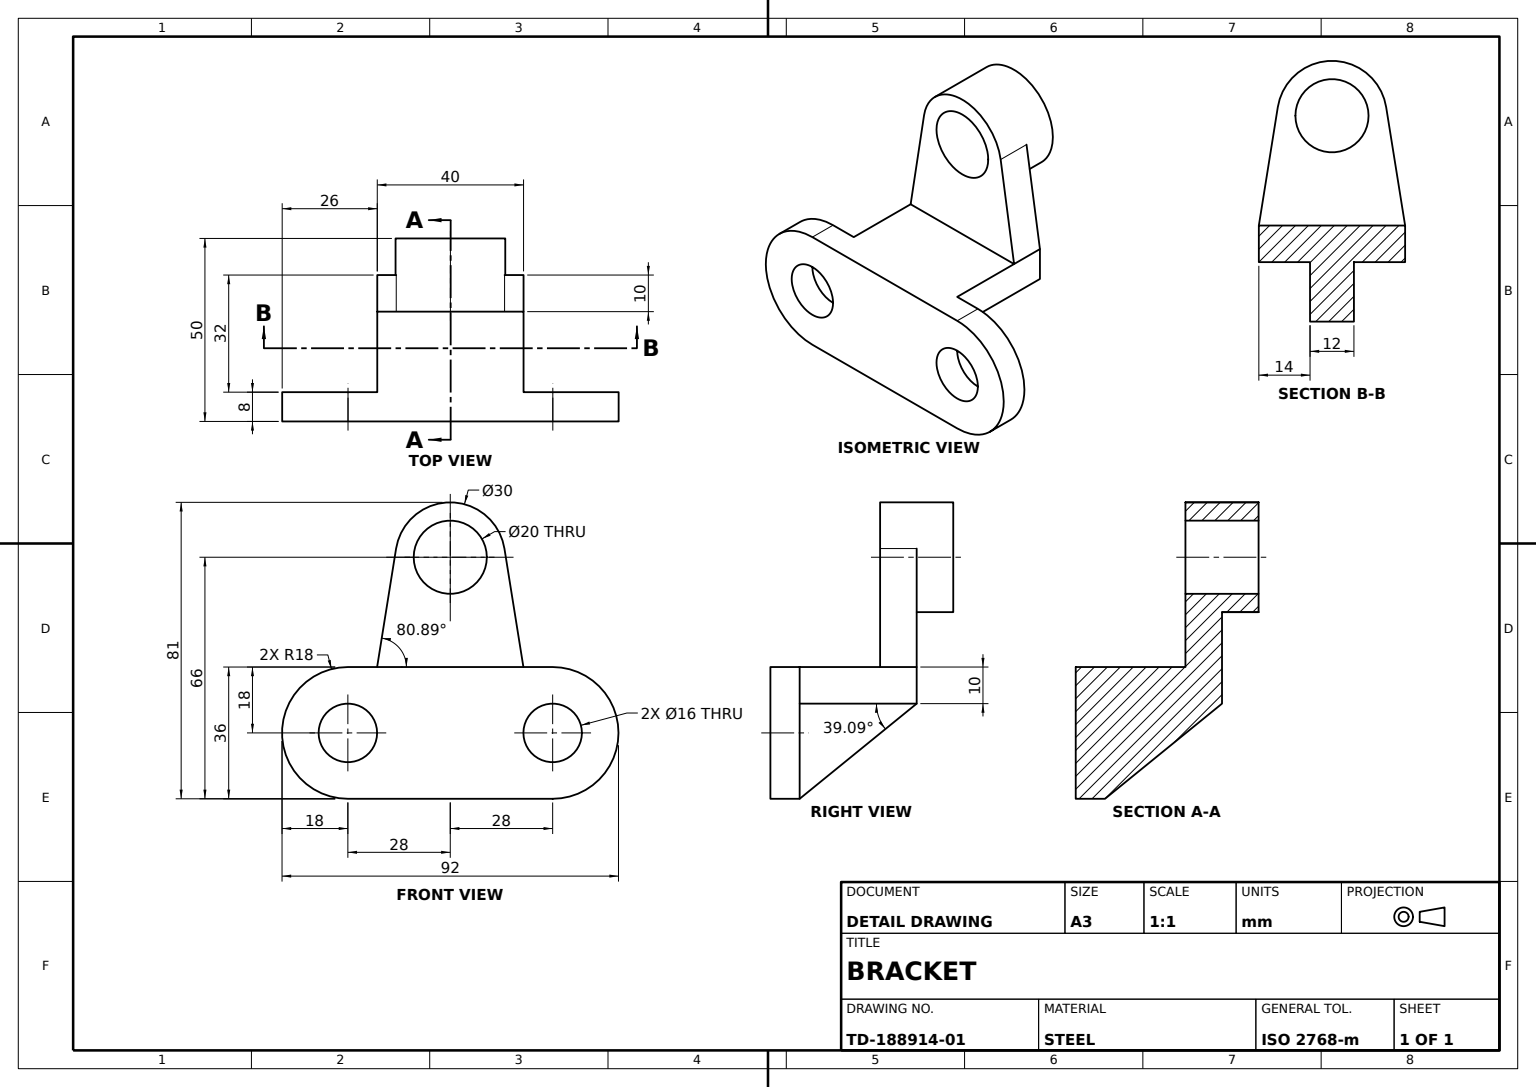
SolidWorks part; units mm, degrees
material "Plain Carbon Steel"
ref_plane "Front Plane" through (0, 0, 0) normal (0, 0, 1) x (1, 0, 0)
ref_plane "Top Plane" through (0, 0, 0) normal (0, 1, 0) x (1, 0, 0)
ref_plane "Right Plane" through (0, 0, 0) normal (1, 0, 0) x (0, 0, -1)
sketch "Base Plate Sketch" plane through (0, 0, 0) normal (0, 0, 1) x (1, 0, 0)
  line L0 (0, 0) -> (92, 0)
  line L1 (0, 0) -> (0, 36)
  line L2 (0, 36) -> (92, 36)
  line L3 (92, 36) -> (92, 0)
  dimension "D1" = 92
  dimension "D2" = 36
extrude "Base Plate" add sketch "Base Plate Sketch" along normal blind 8
sketch "Rounded Ends Sketch" plane through (0, 0, 8) normal (0, 0, 1) x (1, 0, 0)
  line L0 (0, 36) -> (18, 36)
  line L2 (0, 36) -> (0, 0)
  line L6 (0, 0) -> (18, 0)
  line L7 (74, 36) -> (92, 36)
  line L8 (92, 36) -> (92, 0)
  line L9 (92, 0) -> (74, 0)
  arc A0 (18, 36) -> (18, 0) centre (18, 18) ccw
  arc A1 (74, 0) -> (74, 36) centre (74, 18) ccw
  line M3 (0, 36) -> (0, 0)
  line M4 (0, 0) -> (92, 0)
  line M5 (92, 0) -> (92, 36)
  line M6 (92, 36) -> (0, 36)
  dimension "D2" = 18
  dimension "D4" = 18
  dimension "D1" = 18
extrude "Rounded Ends R18" cut sketch "Rounded Ends Sketch" against normal blind 8 contours A0 M6 M3 | A0 L2 M4 | A1 M4 M5 | A1 L8 M6
sketch "Upright Leg Sketch" plane through (0, 36, 0) normal (0, 1, 0) x (1, 0, 0)
  line L0 (46, 0) -> (26, 0)
  line L1 (74, 0) -> (18, 0) construction
  line L2 (26, 0) -> (26, 32)
  line L3 (26, 32) -> (66, 32)
  line L4 (66, 32) -> (66, 0)
  line L5 (66, 0) -> (46, 0)
  dimension "D1" = 20
  dimension "D2" = 32
  dimension "D3" = 40
extrude "Upright Leg" add sketch "Upright Leg Sketch" against normal blind 10
sketch "Lug Head Sketch" plane through (0, 0, -32) normal (0, 0, -1) x (-1, 0, 0)
  line L0 (-46, 36) -> (-46, 66)
  line L1 (-66, 36) -> (-26, 36) construction
  line L2 (-66, 36) -> (-60.811, 68.374)
  line L3 (-26, 36) -> (-31.189, 68.374)
  line L4 (-66, 36) -> (-26, 36)
  circle A0 centre (-46, 66) radius 15
  dimension "D2" = 30
  dimension "D1" = 30
extrude "Lug Head" add sketch "Lug Head Sketch" against normal blind 10
sketch "Round Boss Sketch" plane through (0, 0, -32) normal (0, 0, -1) x (-1, 0, 0)
  circle A0 centre (-46, 66) radius 15
  dimension "D1" = 30
extrude "Raised Round Boss Ø30" add sketch "Round Boss Sketch" along normal blind 10
sketch "Boss Bore Sketch" plane through (0, 0, -42) normal (0, 0, -1) x (-1, 0, 0)
  circle A0 centre (-46, 66) radius 10
  dimension "D1" = 20
extrude "Boss Bore Ø20" cut sketch "Boss Bore Sketch" against normal blind 20
sketch "Mounting Holes Sketch" plane through (0, 0, 0) normal (0, 0, -1) x (-1, 0, 0)
  circle A0 centre (-74, 18) radius 8
  circle A1 centre (-18, 18) radius 8
  dimension "D1" = 16
  dimension "D2" = 16
extrude "Mounting Holes 2xØ16" cut sketch "Mounting Holes Sketch" against normal blind 20
sketch "Rib Sketch" plane through (26, 0, 0) normal (-1, 0, 0) x (0, 0, 1)
  line L0 (-32, 26) -> (0, 26)
  line L1 (0, 26) -> (0, 0)
  line L2 (0, 0) -> (-32, 26)
extrude "Rib" add sketch "Rib Sketch" against normal blind 40
sketch "Rib Trim Sketch 1" plane through (26, 0, 0) normal (-1, 0, 0) x (0, 0, 1)
  line L0 (-32, 26) -> (0, 26)
  line L1 (0, 26) -> (0, 0)
  line L2 (0, 0) -> (-32, 26)
extrude "Rib Trim Cut 1" cut sketch "Rib Trim Sketch 1" against normal blind 14
sketch "Rib Trim Sketch 2" plane through (66, 0, 0) normal (1, 0, 0) x (0, 0, -1)
  line L0 (32, 26) -> (0, 26)
  line L1 (0, 26) -> (0, 0)
  line L2 (0, 0) -> (32, 26)
extrude "Rib Trim Cut 2" cut sketch "Rib Trim Sketch 2" against normal blind 14
